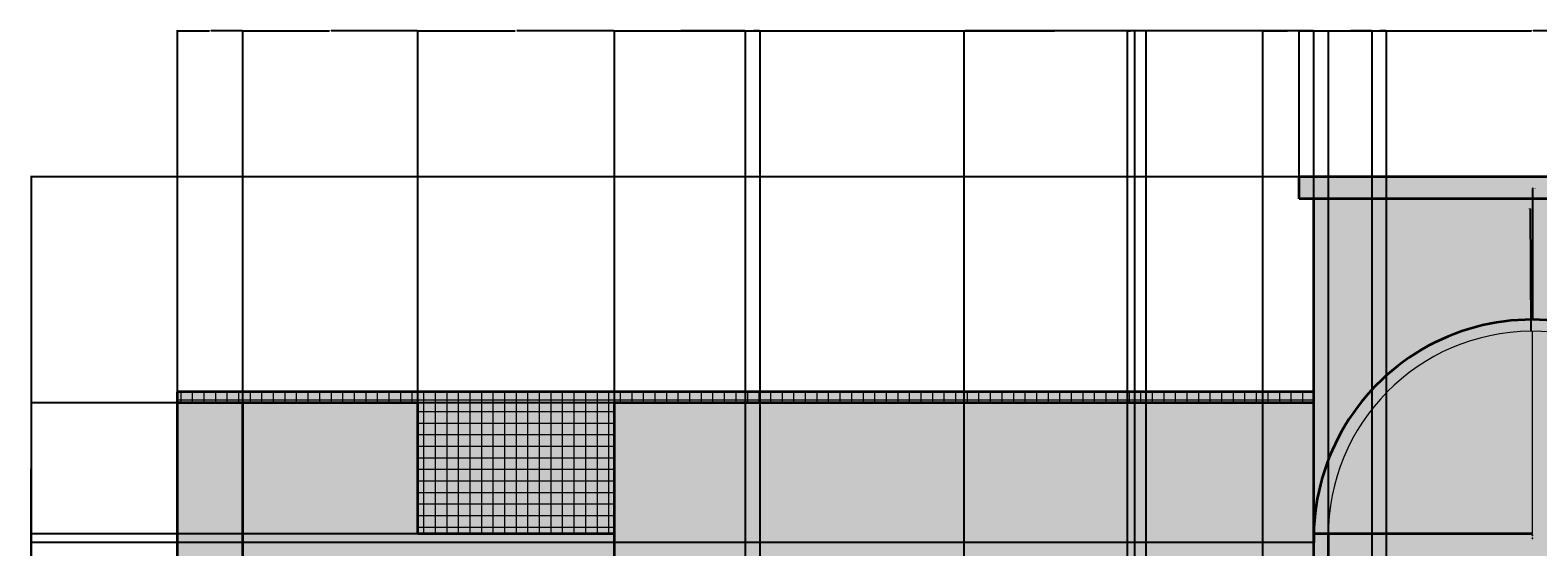
# Model space of a CAD drawing. Units: inches. Extents: x 2794 to 3619, y 522 to 1397.
# Tile 8 of 10: x 2794 to 3208, y 1255 to 1397. Entities that reach past the tile are written whole.
import ezdxf

# ---------------------------------------------------------------- set-up
doc = ezdxf.new("R2010")
doc.units = ezdxf.units.IN
for name, color, linetype, lineweight in [('A-ANNO-DIMS', 2, 'Continuous', 18), ('A-ELEV', 7, 'Continuous', 35), ('A-ELEV-PATT', 8, 'Continuous', 13), ('A-GLAZ', 4, 'Continuous', 18)]:
    doc.layers.add(name, color=color, linetype=linetype, lineweight=lineweight)
doc.styles.get("Standard").update_dxf_attribs({"font": 'arial.ttf'})
doc.dimstyles.get("Standard").update_dxf_attribs({"dimtxt": 0.18, "dimasz": 0.18, "dimexe": 0.18, "dimexo": 0.0625, "dimgap": 0.09, "dimtad": 0, "dimtih": 1, "dimtoh": 1, "dimdec": 4, "dimzin": 0, "dimdsep": 46, "dimtxsty": 'Standard', "dimcen": 0.09, "dimadec": 0, "dimazin": 0, "dimtfac": 1, "dimtdec": 4, "dimtofl": 0, "dimtmove": 0, "dimatfit": 3, "dimfxl": 1, "dimtolj": 1, "dimtzin": 0, "dimarcsym": 0})

# ---------------------------------------------------------------- blocks, each defined once
blk = doc.blocks.new('*D8')
at = {"layer": 'A-ANNO-DIMS', "color": 0, "lineweight": -2, "transparency": 16777216}
for p, q in [((2834.27, 1294.7), (2834.27, 1396.92)), ((2834.45, 1396.74), (2843.06, 1396.74)), ((2852.09, 1396.74), (2843.48, 1396.74)), ((2852.27, 1294.7), (2852.27, 1396.92))]:
    blk.add_line(p, q, dxfattribs=at)
at = {"layer": 'A-ANNO-DIMS', "color": 0, "transparency": 16777216}
for points in [[(2834.45, 1396.77), (2834.45, 1396.71), (2834.27, 1396.74)], [(2852.09, 1396.77), (2852.09, 1396.71), (2852.27, 1396.74)]]:
    blk.add_solid(points, dxfattribs=at)
at = {"layer": 'Defpoints', "color": 0, "transparency": 16777216}
for p in [(2852.27, 1396.74), (2834.27, 1294.64), (2852.27, 1294.64)]:
    blk.add_point(p, dxfattribs=at)
at = {"layer": 'A-ANNO-DIMS', "color": 0, "transparency": 16777216, "insert": (2843.27, 1396.74), "char_height": 0.18, "attachment_point": 5}
blk.add_mtext('\\A1;18', dxfattribs=at)
blk = doc.blocks.new('*D9')
at = {"layer": 'A-ANNO-DIMS', "color": 0, "lineweight": -2, "transparency": 16777216}
for p, q in [((2852.27, 1294.7), (2852.27, 1396.92)), ((2852.45, 1396.74), (2876.04, 1396.74)), ((2900.09, 1396.74), (2876.49, 1396.74)), ((2900.27, 1294.7), (2900.27, 1396.92))]:
    blk.add_line(p, q, dxfattribs=at)
at = {"layer": 'A-ANNO-DIMS', "color": 0, "transparency": 16777216}
for points in [[(2852.45, 1396.77), (2852.45, 1396.71), (2852.27, 1396.74)], [(2900.09, 1396.77), (2900.09, 1396.71), (2900.27, 1396.74)]]:
    blk.add_solid(points, dxfattribs=at)
at = {"layer": 'Defpoints', "color": 0, "transparency": 16777216}
for p in [(2900.27, 1396.74), (2852.27, 1294.64), (2900.27, 1294.64)]:
    blk.add_point(p, dxfattribs=at)
at = {"layer": 'A-ANNO-DIMS', "color": 0, "transparency": 16777216, "insert": (2876.27, 1396.74), "char_height": 0.18, "attachment_point": 5}
blk.add_mtext('\\A1;48', dxfattribs=at)
blk = doc.blocks.new('*D10')
at = {"layer": 'A-ANNO-DIMS', "color": 0, "lineweight": -2, "transparency": 16777216}
for p, q in [((2900.27, 1294.7), (2900.27, 1396.92)), ((2900.45, 1396.74), (2927.05, 1396.74)), ((2954.09, 1396.74), (2927.48, 1396.74)), ((2954.27, 1294.7), (2954.27, 1396.92))]:
    blk.add_line(p, q, dxfattribs=at)
at = {"layer": 'A-ANNO-DIMS', "color": 0, "transparency": 16777216}
for points in [[(2900.45, 1396.77), (2900.45, 1396.71), (2900.27, 1396.74)], [(2954.09, 1396.77), (2954.09, 1396.71), (2954.27, 1396.74)]]:
    blk.add_solid(points, dxfattribs=at)
at = {"layer": 'Defpoints', "color": 0, "transparency": 16777216}
for p in [(2954.27, 1396.74), (2900.27, 1294.64), (2954.27, 1294.64)]:
    blk.add_point(p, dxfattribs=at)
at = {"layer": 'A-ANNO-DIMS', "color": 0, "transparency": 16777216, "insert": (2927.27, 1396.74), "char_height": 0.18, "attachment_point": 5}
blk.add_mtext('\\A1;54', dxfattribs=at)
blk = doc.blocks.new('*D11')
at = {"layer": 'A-ANNO-DIMS', "color": 0, "lineweight": -2, "transparency": 16777216}
for p, q in [((2954.27, 1294.7), (2954.27, 1396.92)), ((2954.45, 1396.74), (3049.99, 1396.74)), ((3146.09, 1396.74), (3050.55, 1396.74)), ((3146.27, 1294.7), (3146.27, 1396.92))]:
    blk.add_line(p, q, dxfattribs=at)
at = {"layer": 'A-ANNO-DIMS', "color": 0, "transparency": 16777216}
for points in [[(2954.45, 1396.77), (2954.45, 1396.71), (2954.27, 1396.74)], [(3146.09, 1396.77), (3146.09, 1396.71), (3146.27, 1396.74)]]:
    blk.add_solid(points, dxfattribs=at)
at = {"layer": 'Defpoints', "color": 0, "transparency": 16777216}
for p in [(3146.27, 1396.74), (2954.27, 1294.64), (3146.27, 1294.64)]:
    blk.add_point(p, dxfattribs=at)
at = {"layer": 'A-ANNO-DIMS', "color": 0, "transparency": 16777216, "insert": (3050.27, 1396.74), "char_height": 0.18, "attachment_point": 5}
blk.add_mtext('\\A1;192', dxfattribs=at)
blk = doc.blocks.new('*D16')
at = {"layer": 'A-ANNO-DIMS', "color": 0, "lineweight": -2, "transparency": 16777216}
for p, q in [((3142.2, 1356.64), (2793.99, 1356.64)), ((2794.17, 1356.46), (2794.17, 959.82)), ((2794.17, 562.82), (2794.17, 959.45)), ((2834.2, 562.64), (2793.99, 562.64))]:
    blk.add_line(p, q, dxfattribs=at)
at = {"layer": 'A-ANNO-DIMS', "color": 0, "transparency": 16777216}
for points in [[(2794.14, 1356.46), (2794.2, 1356.46), (2794.17, 1356.64)], [(2794.14, 562.82), (2794.2, 562.82), (2794.17, 562.64)]]:
    blk.add_solid(points, dxfattribs=at)
at = {"layer": 'Defpoints', "color": 0, "transparency": 16777216}
for p in [(2794.17, 1356.64), (3142.27, 1356.64), (2834.27, 562.64)]:
    blk.add_point(p, dxfattribs=at)
at = {"layer": 'A-ANNO-DIMS', "color": 0, "transparency": 16777216, "insert": (2794.17, 959.64), "char_height": 0.18, "attachment_point": 5}
blk.add_mtext('\\A1;794', dxfattribs=at)
blk = doc.blocks.new('*D26')
at = {"layer": 'A-ANNO-DIMS', "color": 0, "lineweight": -2, "transparency": 16777216}
for p, q in [((2900.2, 1294.64), (2793.99, 1294.64)), ((2794.17, 1294.46), (2794.17, 1276.82)), ((2794.17, 1258.82), (2794.17, 1276.45)), ((2900.2, 1258.64), (2793.99, 1258.64))]:
    blk.add_line(p, q, dxfattribs=at)
at = {"layer": 'A-ANNO-DIMS', "color": 0, "transparency": 16777216}
for points in [[(2794.14, 1294.46), (2794.2, 1294.46), (2794.17, 1294.64)], [(2794.14, 1258.82), (2794.2, 1258.82), (2794.17, 1258.64)]]:
    blk.add_solid(points, dxfattribs=at)
at = {"layer": 'Defpoints', "color": 0, "transparency": 16777216}
for p in [(2794.17, 1294.64), (2900.27, 1294.64), (2900.27, 1258.64)]:
    blk.add_point(p, dxfattribs=at)
at = {"layer": 'A-ANNO-DIMS', "color": 0, "transparency": 16777216, "insert": (2794.17, 1276.64), "char_height": 0.18, "attachment_point": 5}
blk.add_mtext('\\A1;36', dxfattribs=at)
blk = doc.blocks.new('*D27')
at = {"layer": 'A-ANNO-DIMS', "color": 0, "lineweight": -2, "transparency": 16777216}
for p, q in [((2954.2, 1294.64), (2793.99, 1294.64)), ((2794.17, 1294.46), (2794.17, 1261.82)), ((2794.17, 1228.82), (2794.17, 1261.45)), ((2954.2, 1228.64), (2793.99, 1228.64))]:
    blk.add_line(p, q, dxfattribs=at)
at = {"layer": 'A-ANNO-DIMS', "color": 0, "transparency": 16777216}
for points in [[(2794.14, 1294.46), (2794.2, 1294.46), (2794.17, 1294.64)], [(2794.14, 1228.82), (2794.2, 1228.82), (2794.17, 1228.64)]]:
    blk.add_solid(points, dxfattribs=at)
at = {"layer": 'Defpoints', "color": 0, "transparency": 16777216}
for p in [(2794.17, 1294.64), (2954.27, 1294.64), (2954.27, 1228.64)]:
    blk.add_point(p, dxfattribs=at)
at = {"layer": 'A-ANNO-DIMS', "color": 0, "transparency": 16777216, "insert": (2794.17, 1261.64), "char_height": 0.18, "attachment_point": 5}
blk.add_mtext('\\A1;66', dxfattribs=at)
blk = doc.blocks.new('*D28')
at = {"layer": 'A-ANNO-DIMS', "color": 0, "lineweight": -2, "transparency": 16777216}
for p, q in [((2954.27, 832.7), (2954.27, 1396.92)), ((2954.45, 1396.74), (2972.05, 1396.74)), ((2990.09, 1396.74), (2972.48, 1396.74)), ((2990.27, 820.7), (2990.27, 1396.92))]:
    blk.add_line(p, q, dxfattribs=at)
at = {"layer": 'A-ANNO-DIMS', "color": 0, "transparency": 16777216}
for points in [[(2954.45, 1396.77), (2954.45, 1396.71), (2954.27, 1396.74)], [(2990.09, 1396.77), (2990.09, 1396.71), (2990.27, 1396.74)]]:
    blk.add_solid(points, dxfattribs=at)
at = {"layer": 'Defpoints', "color": 0, "transparency": 16777216}
for p in [(2990.27, 1396.74), (2954.27, 832.64), (2990.27, 820.64)]:
    blk.add_point(p, dxfattribs=at)
at = {"layer": 'A-ANNO-DIMS', "color": 0, "transparency": 16777216, "insert": (2972.27, 1396.74), "char_height": 0.18, "attachment_point": 5}
blk.add_mtext('\\A1;36', dxfattribs=at)
blk = doc.blocks.new('*D29')
at = {"layer": 'A-ANNO-DIMS', "color": 0, "lineweight": -2, "transparency": 16777216}
for p, q in [((2990.27, 820.7), (2990.27, 1396.92)), ((2990.45, 1396.74), (2992.11, 1396.74)), ((2994.09, 1396.74), (2992.42, 1396.74)), ((2994.27, 816.7), (2994.27, 1396.92))]:
    blk.add_line(p, q, dxfattribs=at)
at = {"layer": 'A-ANNO-DIMS', "color": 0, "transparency": 16777216}
for points in [[(2990.45, 1396.77), (2990.45, 1396.71), (2990.27, 1396.74)], [(2994.09, 1396.77), (2994.09, 1396.71), (2994.27, 1396.74)]]:
    blk.add_solid(points, dxfattribs=at)
at = {"layer": 'Defpoints', "color": 0, "transparency": 16777216}
for p in [(2994.27, 1396.74), (2990.27, 820.64), (2994.27, 816.64)]:
    blk.add_point(p, dxfattribs=at)
at = {"layer": 'A-ANNO-DIMS', "color": 0, "transparency": 16777216, "insert": (2992.27, 1396.74), "char_height": 0.18, "attachment_point": 5}
blk.add_mtext('\\A1;4', dxfattribs=at)
blk = doc.blocks.new('*D30')
at = {"layer": 'A-ANNO-DIMS', "color": 0, "lineweight": -2, "transparency": 16777216}
for p, q in [((3050.27, 820.7), (3050.27, 1396.92)), ((3050.45, 1396.74), (3075.05, 1396.74)), ((3100.09, 1396.74), (3075.48, 1396.74)), ((3100.27, 820.7), (3100.27, 1396.92))]:
    blk.add_line(p, q, dxfattribs=at)
at = {"layer": 'A-ANNO-DIMS', "color": 0, "transparency": 16777216}
for points in [[(3050.45, 1396.77), (3050.45, 1396.71), (3050.27, 1396.74)], [(3100.09, 1396.77), (3100.09, 1396.71), (3100.27, 1396.74)]]:
    blk.add_solid(points, dxfattribs=at)
at = {"layer": 'Defpoints', "color": 0, "transparency": 16777216}
for p in [(3100.27, 1396.74), (3050.27, 820.64), (3100.27, 820.64)]:
    blk.add_point(p, dxfattribs=at)
at = {"layer": 'A-ANNO-DIMS', "color": 0, "transparency": 16777216, "insert": (3075.27, 1396.74), "char_height": 0.18, "attachment_point": 5}
blk.add_mtext('\\A1;50', dxfattribs=at)
blk = doc.blocks.new('*D31')
at = {"layer": 'A-ANNO-DIMS', "color": 0, "lineweight": -2, "transparency": 16777216}
for p, q in [((3132.27, 820.7), (3132.27, 1396.92)), ((3132.45, 1396.74), (3139.06, 1396.74)), ((3146.09, 1396.74), (3139.48, 1396.74)), ((3146.27, 774.7), (3146.27, 1396.92))]:
    blk.add_line(p, q, dxfattribs=at)
at = {"layer": 'A-ANNO-DIMS', "color": 0, "transparency": 16777216}
for points in [[(3132.45, 1396.77), (3132.45, 1396.71), (3132.27, 1396.74)], [(3146.09, 1396.77), (3146.09, 1396.71), (3146.27, 1396.74)]]:
    blk.add_solid(points, dxfattribs=at)
at = {"layer": 'Defpoints', "color": 0, "transparency": 16777216}
for p in [(3146.27, 1396.74), (3132.27, 820.64), (3146.27, 774.64)]:
    blk.add_point(p, dxfattribs=at)
at = {"layer": 'A-ANNO-DIMS', "color": 0, "transparency": 16777216, "insert": (3139.27, 1396.74), "char_height": 0.18, "attachment_point": 5}
blk.add_mtext('\\A1;14', dxfattribs=at)
blk = doc.blocks.new('*D37')
at = {"layer": 'A-ANNO-DIMS', "color": 0, "lineweight": -2, "transparency": 16777216}
for p, q in [((3095.13, 772.7), (3095.13, 1396.92)), ((3095.31, 1396.74), (3095.98, 1396.74)), ((3096.95, 1396.74), (3096.28, 1396.74)), ((3097.13, 772.7), (3097.13, 1396.92))]:
    blk.add_line(p, q, dxfattribs=at)
at = {"layer": 'A-ANNO-DIMS', "color": 0, "transparency": 16777216}
for points in [[(3095.31, 1396.77), (3095.31, 1396.71), (3095.13, 1396.74)], [(3096.95, 1396.77), (3096.95, 1396.71), (3097.13, 1396.74)]]:
    blk.add_solid(points, dxfattribs=at)
at = {"layer": 'Defpoints', "color": 0, "transparency": 16777216}
for p in [(3097.13, 1396.74), (3095.13, 772.64), (3097.13, 772.64)]:
    blk.add_point(p, dxfattribs=at)
at = {"layer": 'A-ANNO-DIMS', "color": 0, "transparency": 16777216, "insert": (3096.13, 1396.74), "char_height": 0.18, "attachment_point": 5}
blk.add_mtext('\\A1;2', dxfattribs=at)
blk = doc.blocks.new('*D44')
at = {"layer": 'A-ANNO-DIMS', "color": 0, "lineweight": -2, "transparency": 16777216}
for p, q in [((3142.27, 1356.7), (3142.27, 1396.92)), ((3142.45, 1396.74), (3205.99, 1396.74)), ((3270.09, 1396.74), (3206.55, 1396.74)), ((3270.27, 1356.7), (3270.27, 1396.92))]:
    blk.add_line(p, q, dxfattribs=at)
at = {"layer": 'A-ANNO-DIMS', "color": 0, "transparency": 16777216}
for points in [[(3142.45, 1396.77), (3142.45, 1396.71), (3142.27, 1396.74)], [(3270.09, 1396.77), (3270.09, 1396.71), (3270.27, 1396.74)]]:
    blk.add_solid(points, dxfattribs=at)
at = {"layer": 'Defpoints', "color": 0, "transparency": 16777216}
for p in [(3270.27, 1396.74), (3142.27, 1356.64), (3270.27, 1356.64)]:
    blk.add_point(p, dxfattribs=at)
at = {"layer": 'A-ANNO-DIMS', "color": 0, "transparency": 16777216, "insert": (3206.27, 1396.74), "char_height": 0.18, "attachment_point": 5}
blk.add_mtext('\\A1;128', dxfattribs=at)
blk = doc.blocks.new('*D45')
at = {"layer": 'A-ANNO-DIMS', "color": 0, "lineweight": -2, "transparency": 16777216}
for p, q in [((3146.27, 1350.7), (3146.27, 1396.92)), ((3146.45, 1396.74), (3205.99, 1396.74)), ((3266.09, 1396.74), (3206.55, 1396.74)), ((3266.27, 1350.7), (3266.27, 1396.92))]:
    blk.add_line(p, q, dxfattribs=at)
at = {"layer": 'A-ANNO-DIMS', "color": 0, "transparency": 16777216}
for points in [[(3146.45, 1396.77), (3146.45, 1396.71), (3146.27, 1396.74)], [(3266.09, 1396.77), (3266.09, 1396.71), (3266.27, 1396.74)]]:
    blk.add_solid(points, dxfattribs=at)
at = {"layer": 'Defpoints', "color": 0, "transparency": 16777216}
for p in [(3266.27, 1396.74), (3146.27, 1350.64), (3266.27, 1350.64)]:
    blk.add_point(p, dxfattribs=at)
at = {"layer": 'A-ANNO-DIMS', "color": 0, "transparency": 16777216, "insert": (3206.27, 1396.74), "char_height": 0.18, "attachment_point": 5}
blk.add_mtext('\\A1;120', dxfattribs=at)
blk = doc.blocks.new('*D48')
at = {"layer": 'A-ANNO-DIMS', "color": 0, "lineweight": -2, "transparency": 16777216}
for p, q in [((3146.2, 1294.64), (2793.99, 1294.64)), ((2794.17, 1294.46), (2794.17, 1275.62)), ((2794.17, 1256.43), (2794.17, 1275.26)), ((3146.2, 1256.25), (2793.99, 1256.25))]:
    blk.add_line(p, q, dxfattribs=at)
at = {"layer": 'A-ANNO-DIMS', "color": 0, "transparency": 16777216}
for points in [[(2794.14, 1294.46), (2794.2, 1294.46), (2794.17, 1294.64)], [(2794.14, 1256.43), (2794.2, 1256.43), (2794.17, 1256.25)]]:
    blk.add_solid(points, dxfattribs=at)
at = {"layer": 'Defpoints', "color": 0, "transparency": 16777216}
for p in [(2794.17, 1294.64), (3146.27, 1294.64), (3146.27, 1256.25)]:
    blk.add_point(p, dxfattribs=at)
at = {"layer": 'A-ANNO-DIMS', "color": 0, "transparency": 16777216, "insert": (2794.17, 1275.44), "char_height": 0.18, "attachment_point": 5}
blk.add_mtext('\\A1;38.39', dxfattribs=at)
blk = doc.blocks.new('*D49')
at = {"layer": 'A-ANNO-DIMS', "color": 0, "lineweight": -2, "transparency": 16777216}
for p, q in [((3146.27, 1256.19), (3146.27, 522.36)), ((3150.27, 1254.57), (3150.27, 522.36)), ((3146.45, 522.54), (3148.11, 522.54)), ((3150.09, 522.54), (3148.42, 522.54))]:
    blk.add_line(p, q, dxfattribs=at)
at = {"layer": 'A-ANNO-DIMS', "color": 0, "transparency": 16777216}
for points in [[(3146.45, 522.57), (3146.45, 522.51), (3146.27, 522.54)], [(3150.09, 522.57), (3150.09, 522.51), (3150.27, 522.54)]]:
    blk.add_solid(points, dxfattribs=at)
at = {"layer": 'Defpoints', "color": 0, "transparency": 16777216}
for p in [(3146.27, 1256.25), (3150.27, 1254.64), (3150.27, 522.54)]:
    blk.add_point(p, dxfattribs=at)
at = {"layer": 'A-ANNO-DIMS', "color": 0, "transparency": 16777216, "insert": (3148.27, 522.54), "char_height": 0.18, "attachment_point": 5}
blk.add_mtext('\\A1;4', dxfattribs=at)
blk = doc.blocks.new('*D56')
at = {"layer": 'A-ANNO-DIMS', "color": 0, "lineweight": -2, "transparency": 16777216}
for p, q in [((3162.27, 664.7), (3162.27, 1396.92)), ((3162.45, 1396.74), (3206.05, 1396.74)), ((3250.09, 1396.74), (3206.49, 1396.74)), ((3250.27, 664.7), (3250.27, 1396.92))]:
    blk.add_line(p, q, dxfattribs=at)
at = {"layer": 'A-ANNO-DIMS', "color": 0, "transparency": 16777216}
for points in [[(3162.45, 1396.77), (3162.45, 1396.71), (3162.27, 1396.74)], [(3250.09, 1396.77), (3250.09, 1396.71), (3250.27, 1396.74)]]:
    blk.add_solid(points, dxfattribs=at)
at = {"layer": 'Defpoints', "color": 0, "transparency": 16777216}
for p in [(3250.27, 1396.74), (3162.27, 664.64), (3250.27, 664.64)]:
    blk.add_point(p, dxfattribs=at)
at = {"layer": 'A-ANNO-DIMS', "color": 0, "transparency": 16777216, "insert": (3206.27, 1396.74), "char_height": 0.18, "attachment_point": 5}
blk.add_mtext('\\A1;88', dxfattribs=at)
blk = doc.blocks.new('*D57')
at = {"layer": 'A-ANNO-DIMS', "color": 0, "lineweight": -2, "transparency": 16777216}
for p, q in [((3162.27, 664.7), (3162.27, 1396.92)), ((3162.45, 1396.74), (3164.11, 1396.74)), ((3166.09, 1396.74), (3164.42, 1396.74)), ((3166.27, 660.7), (3166.27, 1396.92))]:
    blk.add_line(p, q, dxfattribs=at)
at = {"layer": 'A-ANNO-DIMS', "color": 0, "transparency": 16777216}
for points in [[(3162.45, 1396.77), (3162.45, 1396.71), (3162.27, 1396.74)], [(3166.09, 1396.77), (3166.09, 1396.71), (3166.27, 1396.74)]]:
    blk.add_solid(points, dxfattribs=at)
at = {"layer": 'Defpoints', "color": 0, "transparency": 16777216}
for p in [(3166.27, 1396.74), (3162.27, 664.64), (3166.27, 660.64)]:
    blk.add_point(p, dxfattribs=at)
at = {"layer": 'A-ANNO-DIMS', "color": 0, "transparency": 16777216, "insert": (3164.27, 1396.74), "char_height": 0.18, "attachment_point": 5}
blk.add_mtext('\\A1;4', dxfattribs=at)
blk = doc.blocks.new('*D58')
at = {"layer": 'A-ANNO-DIMS', "color": 0, "lineweight": -2, "transparency": 16777216}
for p, q in [((3150.27, 580.7), (3150.27, 1396.92)), ((3150.45, 1396.74), (3156.06, 1396.74)), ((3162.09, 1396.74), (3156.48, 1396.74)), ((3162.27, 664.7), (3162.27, 1396.92))]:
    blk.add_line(p, q, dxfattribs=at)
at = {"layer": 'A-ANNO-DIMS', "color": 0, "transparency": 16777216}
for points in [[(3150.45, 1396.77), (3150.45, 1396.71), (3150.27, 1396.74)], [(3162.09, 1396.77), (3162.09, 1396.71), (3162.27, 1396.74)]]:
    blk.add_solid(points, dxfattribs=at)
at = {"layer": 'Defpoints', "color": 0, "transparency": 16777216}
for p in [(3162.27, 1396.74), (3162.27, 664.64), (3150.27, 580.64)]:
    blk.add_point(p, dxfattribs=at)
at = {"layer": 'A-ANNO-DIMS', "color": 0, "transparency": 16777216, "insert": (3156.27, 1396.74), "char_height": 0.18, "attachment_point": 5}
blk.add_mtext('\\A1;12', dxfattribs=at)
blk = doc.blocks.new('*D64')
at = {"layer": 'A-ANNO-DIMS', "color": 0, "lineweight": -2, "transparency": 16777216}
for p, q in [((3206.45, 1353.46), (3206.27, 1353.46)), ((3206.27, 1353.46), (3206.27, 1317.63)), ((3206.18, 1257.44), (3206.36, 1257.44)), ((3206.27, 1257.35), (3206.27, 1257.53))]:
    blk.add_line(p, q, dxfattribs=at)
at = {"layer": 'A-ANNO-DIMS', "color": 0, "transparency": 16777216}
blk.add_solid([(3206.24, 1317.63), (3206.3, 1317.63), (3206.27, 1317.45)], dxfattribs=at)
at = {"layer": 'Defpoints', "color": 0, "transparency": 16777216}
for p in [(3206.27, 1317.45), (3206.27, 1257.44)]:
    blk.add_point(p, dxfattribs=at)
at = {"layer": 'A-ANNO-DIMS', "color": 0, "transparency": 16777216, "insert": (3206.91, 1353.46), "char_height": 0.18, "attachment_point": 5}
blk.add_mtext('\\A1;R60.01', dxfattribs=at)
blk = doc.blocks.new('*D65')
at = {"layer": 'A-ANNO-DIMS', "color": 0, "lineweight": -2, "transparency": 16777216}
for p, q in [((3205.48, 1347.85), (3205.66, 1347.85)), ((3205.66, 1347.85), (3205.88, 1314.43)), ((3206.27, 1258.16), (3206.27, 1258.34)), ((3206.18, 1258.25), (3206.36, 1258.25))]:
    blk.add_line(p, q, dxfattribs=at)
at = {"layer": 'A-ANNO-DIMS', "color": 0, "transparency": 16777216}
blk.add_solid([(3205.91, 1314.43), (3205.85, 1314.43), (3205.89, 1314.25)], dxfattribs=at)
at = {"layer": 'Defpoints', "color": 0, "transparency": 16777216}
for p in [(3205.89, 1314.25), (3206.27, 1258.25)]:
    blk.add_point(p, dxfattribs=at)
at = {"layer": 'A-ANNO-DIMS', "color": 0, "transparency": 16777216, "insert": (3205.17, 1347.85), "char_height": 0.18, "attachment_point": 5}
blk.add_mtext('\\A1;R56', dxfattribs=at)

msp = doc.modelspace()

# ---------------------------------------------------------------- hatches: boundary and pattern name
at = {"layer": 'A-ELEV-PATT', "transparency": 33554687}
h = msp.add_hatch(color=256, dxfattribs=at)
h.dxf.hatch_style = 1
h.paths.add_polyline_path([(3270.2659, 1356.6351), (3142.2659, 1356.6351), (3142.2659, 1350.6351), (3266.2659, 1350.6351), (3270.2659, 1350.6351)])
h.paths.add_polyline_path([(3266.2659, 1350.6351), (3262.2659, 1350.6351), (3262.2659, 1279.0155, -0.0871789), (3266.2659, 1258.6351)])
h.paths.add_polyline_path([(3150.2659, 1350.6351), (3146.2659, 1350.6351), (3146.2659, 1258.6351, -0.0871789), (3150.2659, 1279.0155)])
h = msp.add_hatch(color=256, dxfattribs=at)
h.dxf.hatch_style = 1
h.paths.add_polyline_path([(3262.2659, 1350.6351), (3150.2659, 1350.6351), (3150.2659, 1279.0155, -0.68639605), (3262.2659, 1279.0155)])
h.paths.add_polyline_path([(3210.2659, 1314.1121), (3210.2659, 1258.6351), (3262.2659, 1258.6351, 0.39146256)])
h.paths.add_polyline_path([(3206.2659, 1314.2551, 0.41222069), (3150.2659, 1258.6351), (3206.2659, 1258.6351)])
h.paths.add_polyline_path([(3262.2659, 1254.6351), (3210.2659, 1254.6351), (3210.2659, 1216.6351), (3262.2659, 1216.6351)])
h.paths.add_polyline_path([(3206.2659, 1254.6351), (3150.2659, 1254.6351), (3150.2659, 1216.6351), (3206.2659, 1216.6351)])
h.paths.add_polyline_path([(3262.2659, 1212.6351), (3210.2659, 1212.6351), (3210.2659, 1186.6351), (3262.2659, 1186.6351)])
h.paths.add_polyline_path([(3206.2659, 1212.6351), (3150.2659, 1212.6351), (3150.2659, 1186.6351), (3206.2659, 1186.6351)])
h.paths.add_polyline_path([(3206.2659, 1182.6351), (3150.2659, 1182.6351), (3150.2659, 1156.6351), (3206.2659, 1156.6351)])
h.paths.add_polyline_path([(3262.2659, 1182.6351), (3210.2659, 1182.6351), (3210.2659, 1156.6351), (3262.2659, 1156.6351)])
h.paths.add_polyline_path([(3262.2659, 1152.6351), (3210.2659, 1152.6351), (3210.2659, 1126.6351), (3262.2659, 1126.6351)])
h.paths.add_polyline_path([(3206.2659, 1152.6351), (3150.2659, 1152.6351), (3150.2659, 1126.6351), (3206.2659, 1126.6351)])
h.paths.add_polyline_path([(3262.2659, 1122.6351), (3210.2659, 1122.6351), (3210.2659, 1096.6351), (3262.2659, 1096.6351)])
h.paths.add_polyline_path([(3206.2659, 1122.6351), (3150.2659, 1122.6351), (3150.2659, 1096.6351), (3206.2659, 1096.6351)])
h.paths.add_polyline_path([(3206.2659, 1092.6351), (3150.2659, 1092.6351), (3150.2659, 1066.6351), (3206.2659, 1066.6351)])
h.paths.add_polyline_path([(3262.2659, 1092.6351), (3210.2659, 1092.6351), (3210.2659, 1066.6351), (3262.2659, 1066.6351)])
h.paths.add_polyline_path([(3262.2659, 1062.6351), (3210.2659, 1062.6351), (3210.2659, 1036.6351), (3262.2659, 1036.6351)])
h.paths.add_polyline_path([(3206.2659, 1062.6351), (3150.2659, 1062.6351), (3150.2659, 1036.6351), (3206.2659, 1036.6351)])
h.paths.add_polyline_path([(3206.2659, 1032.6351), (3150.2659, 1032.6351), (3150.2659, 1006.6351), (3206.2659, 1006.6351)])
h.paths.add_polyline_path([(3262.2659, 1032.6351), (3210.2659, 1032.6351), (3210.2659, 1006.6351), (3262.2659, 1006.6351)])
h.paths.add_polyline_path([(3262.2659, 1002.6351), (3210.2659, 1002.6351), (3210.2659, 976.6351), (3262.2659, 976.6351)])
h.paths.add_polyline_path([(3206.2659, 1002.6351), (3150.2659, 1002.6351), (3150.2659, 976.6351), (3206.2659, 976.6351)])
h.paths.add_polyline_path([(3206.2659, 972.6351), (3150.2659, 972.6351), (3150.2659, 946.6351), (3206.2659, 946.6351)])
h.paths.add_polyline_path([(3206.2659, 942.6351), (3150.2659, 942.6351), (3150.2659, 916.6351), (3206.2659, 916.6351)])
h.paths.add_polyline_path([(3262.2659, 942.6351), (3210.2659, 942.6351), (3210.2659, 916.6351), (3262.2659, 916.6351)])
h.paths.add_polyline_path([(3262.2659, 972.6351), (3210.2659, 972.6351), (3210.2659, 946.6351), (3262.2659, 946.6351)])
h.paths.add_polyline_path([(3262.2659, 912.6351), (3210.2659, 912.6351), (3210.2659, 886.6351), (3262.2659, 886.6351)])
h.paths.add_polyline_path([(3206.2659, 912.6351), (3150.2659, 912.6351), (3150.2659, 886.6351), (3206.2659, 886.6351)])
h.paths.add_polyline_path([(3206.2659, 882.6351), (3150.2659, 882.6351), (3150.2659, 856.6351), (3206.2659, 856.6351)])
h.paths.add_polyline_path([(3262.2659, 882.6351), (3210.2659, 882.6351), (3210.2659, 856.6351), (3262.2659, 856.6351)])
h.paths.add_polyline_path([(3262.2659, 852.6351), (3210.2659, 852.6351), (3210.2659, 826.6351), (3262.2659, 826.6351)])
h.paths.add_polyline_path([(3206.2659, 852.6351), (3150.2659, 852.6351), (3150.2659, 826.6351), (3206.2659, 826.6351)])
h.paths.add_polyline_path([(3206.2659, 822.6351), (3150.2659, 822.6351), (3150.2659, 796.6351), (3206.2659, 796.6351)])
h.paths.add_polyline_path([(3262.2659, 822.6351), (3210.2659, 822.6351), (3210.2659, 796.6351), (3262.2659, 796.6351)])
h.paths.add_polyline_path([(3262.2659, 792.6351), (3210.2659, 792.6351), (3210.2659, 766.6351), (3262.2659, 766.6351)])
h.paths.add_polyline_path([(3206.2659, 792.6351), (3150.2659, 792.6351), (3150.2659, 766.6351), (3206.2659, 766.6351)])
h.paths.add_polyline_path([(3206.2659, 762.6351), (3150.2659, 762.6351), (3150.2659, 736.6351), (3206.2659, 736.6351)])
h.paths.add_polyline_path([(3206.2659, 732.6351), (3150.2659, 732.6351), (3150.2659, 706.6351), (3206.2659, 706.6351)])
h.paths.add_polyline_path([(3262.2659, 732.6351), (3210.2659, 732.6351), (3210.2659, 706.6351), (3262.2659, 706.6351)])
h.paths.add_polyline_path([(3262.2659, 762.6351), (3210.2659, 762.6351), (3210.2659, 736.6351), (3262.2659, 736.6351)])
h = msp.add_hatch(color=256, dxfattribs=at)
h.dxf.hatch_style = 1
h.paths.add_polyline_path([(3146.2659, 1258.6351), (3150.2659, 1258.6351, -0.9932142), (3262.2659, 1258.6351), (3262.2659, 1279.0155, 0.82281137)])
h = msp.add_hatch(color=256, dxfattribs=at)
h.dxf.hatch_style = 1
h.paths.add_polyline_path([(3266.2659, 1258.6351, 0.98030963), (3146.2659, 1258.6351), (3150.2659, 1258.6351, -0.9932142), (3262.2659, 1258.6351), (3262.2659, 1228.6351), (3266.2659, 1228.6351)])
h = msp.add_hatch(color=256, dxfattribs=at)
h.dxf.hatch_style = 1
h.paths.add_polyline_path([(3150.2659, 1257.8725, -0.00340445), (3150.2659, 1258.6351), (3146.2659, 1258.6351), (3146.2659, 1228.6351), (3150.2659, 1228.6351)])
h.paths.add_polyline_path([(3262.2659, 1258.6351), (3210.2659, 1258.6351), (3210.2659, 1314.1121, 0.01787385), (3206.2659, 1314.2551), (3206.2659, 1258.6351), (3150.2659, 1258.6351), (3150.2659, 1254.6351), (3206.2659, 1254.6351), (3206.2659, 1216.6351), (3150.2659, 1216.6351), (3150.2659, 1212.6351), (3206.2659, 1212.6351), (3206.2659, 1186.6351), (3150.2659, 1186.6351), (3150.2659, 1182.6351), (3206.2659, 1182.6351), (3206.2659, 1156.6351), (3150.2659, 1156.6351), (3150.2659, 1152.6351), (3206.2659, 1152.6351), (3206.2659, 1126.6351), (3150.2659, 1126.6351), (3150.2659, 1122.6351), (3206.2659, 1122.6351), (3206.2659, 1096.6351), (3150.2659, 1096.6351), (3150.2659, 1092.6351), (3206.2659, 1092.6351), (3206.2659, 1066.6351), (3150.2659, 1066.6351), (3150.2659, 1062.6351), (3206.2659, 1062.6351), (3206.2659, 1036.6351), (3150.2659, 1036.6351), (3150.2659, 1032.6351), (3206.2659, 1032.6351), (3206.2659, 1006.6351), (3150.2659, 1006.6351), (3150.2659, 1002.6351), (3206.2659, 1002.6351), (3206.2659, 976.6351), (3150.2659, 976.6351), (3150.2659, 972.6351), (3206.2659, 972.6351), (3206.2659, 946.6351), (3150.2659, 946.6351), (3150.2659, 942.6351), (3206.2659, 942.6351), (3206.2659, 916.6351), (3150.2659, 916.6351), (3150.2659, 912.6351), (3206.2659, 912.6351), (3206.2659, 886.6351), (3150.2659, 886.6351), (3150.2659, 882.6351), (3206.2659, 882.6351), (3206.2659, 856.6351), (3150.2659, 856.6351), (3150.2659, 852.6351), (3206.2659, 852.6351), (3206.2659, 826.6351), (3150.2659, 826.6351), (3150.2659, 822.6351), (3206.2659, 822.6351), (3206.2659, 796.6351), (3150.2659, 796.6351), (3150.2659, 792.6351), (3206.2659, 792.6351), (3206.2659, 766.6351), (3150.2659, 766.6351), (3150.2659, 762.6351), (3206.2659, 762.6351), (3206.2659, 736.6351), (3150.2659, 736.6351), (3150.2659, 732.6351), (3206.2659, 732.6351), (3206.2659, 706.6351), (3150.2659, 706.6351), (3150.2659, 702.6351), (3262.2659, 702.6351), (3262.2659, 706.6351), (3210.2659, 706.6351), (3210.2659, 732.6351), (3262.2659, 732.6351), (3262.2659, 736.6351), (3210.2659, 736.6351), (3210.2659, 762.6351), (3262.2659, 762.6351), (3262.2659, 766.6351), (3210.2659, 766.6351), (3210.2659, 792.6351), (3262.2659, 792.6351), (3262.2659, 796.6351), (3210.2659, 796.6351), (3210.2659, 822.6351), (3262.2659, 822.6351), (3262.2659, 826.6351), (3210.2659, 826.6351), (3210.2659, 852.6351), (3262.2659, 852.6351), (3262.2659, 856.6351), (3210.2659, 856.6351), (3210.2659, 882.6351), (3262.2659, 882.6351), (3262.2659, 886.6351), (3210.2659, 886.6351), (3210.2659, 912.6351), (3262.2659, 912.6351), (3262.2659, 916.6351), (3210.2659, 916.6351), (3210.2659, 942.6351), (3262.2659, 942.6351), (3262.2659, 946.6351), (3210.2659, 946.6351), (3210.2659, 972.6351), (3262.2659, 972.6351), (3262.2659, 976.6351), (3210.2659, 976.6351), (3210.2659, 1002.6351), (3262.2659, 1002.6351), (3262.2659, 1006.6351), (3210.2659, 1006.6351), (3210.2659, 1032.6351), (3262.2659, 1032.6351), (3262.2659, 1036.6351), (3210.2659, 1036.6351), (3210.2659, 1062.6351), (3262.2659, 1062.6351), (3262.2659, 1066.6351), (3210.2659, 1066.6351), (3210.2659, 1092.6351), (3262.2659, 1092.6351), (3262.2659, 1096.6351), (3210.2659, 1096.6351), (3210.2659, 1122.6351), (3262.2659, 1122.6351), (3262.2659, 1126.6351), (3210.2659, 1126.6351), (3210.2659, 1152.6351), (3262.2659, 1152.6351), (3262.2659, 1156.6351), (3210.2659, 1156.6351), (3210.2659, 1182.6351), (3262.2659, 1182.6351), (3262.2659, 1186.6351), (3210.2659, 1186.6351), (3210.2659, 1212.6351), (3262.2659, 1212.6351), (3262.2659, 1216.6351), (3210.2659, 1216.6351), (3210.2659, 1254.6351), (3262.2659, 1254.6351)])
at = {"layer": 'A-ELEV-PATT'}
h = msp.add_hatch(dxfattribs=at)
h.set_pattern_fill('NET', color=256)
h.paths.add_polyline_path([(2834.2659, 1297.6351), (2834.2659, 1294.6351), (2900.2659, 1294.6351), (2900.2659, 1258.6351), (2954.2659, 1258.6351), (2954.2659, 1294.6351), (3146.2659, 1294.6351), (3146.2659, 1297.6351)])
h.paths.add_polyline_path([(3512.2659, 1258.6351), (3512.2659, 1294.6351), (3578.2659, 1294.6351), (3578.2659, 1297.6351), (3266.2659, 1297.6351), (3266.2659, 1294.6351), (3458.2659, 1294.6351), (3458.2659, 1258.6351)])
at = {"layer": 'A-ELEV-PATT', "transparency": 33554687}
h = msp.add_hatch(color=256, dxfattribs=at)
h.dxf.hatch_style = 1
h.paths.add_polyline_path([(2834.2659, 1297.6351), (2834.2659, 1294.6351), (2900.2659, 1294.6351), (2900.2659, 1258.6351), (2954.2659, 1258.6351), (2954.2659, 1294.6351), (3146.2659, 1294.6351), (3146.2659, 1297.6351)])
h = msp.add_hatch(color=256, dxfattribs=at)
h.dxf.hatch_style = 1
h.paths.add_polyline_path([(3578.2659, 1294.6351), (3560.2659, 1294.6351), (3560.2659, 642.6351), (3578.2659, 642.6351)])
h.paths.add_polyline_path([(2852.2659, 1294.6351), (2834.2659, 1294.6351), (2834.2659, 642.6351), (2852.2659, 642.6351)])
h = msp.add_hatch(color=256, dxfattribs=at)
h.dxf.hatch_style = 1
h.paths.add_polyline_path([(2852.2659, 1294.6351), (2834.2659, 1294.6351), (2834.2659, 562.6351), (2852.2659, 562.6351)])
h.paths.add_polyline_path([(3578.2659, 1294.6351), (3560.2659, 1294.6351), (3560.2659, 562.6351), (3578.2659, 562.6351)])
h = msp.add_hatch(color=256, dxfattribs=at)
h.dxf.hatch_style = 1
h.paths.add_polyline_path([(2852.2659, 1246.6351), (2954.2659, 1246.6351), (2954.2659, 1258.6351), (2900.2659, 1258.6351), (2900.2659, 1294.6351), (2852.2659, 1294.6351)])
h.paths.add_polyline_path([(3512.2659, 1294.6351), (3512.2659, 1258.6351), (3458.2659, 1258.6351), (3458.2659, 1246.6351), (3560.2659, 1246.6351), (3560.2659, 1294.6351)])
h.paths.add_polyline_path([(2954.2659, 1114.6351), (2954.2659, 1126.6351), (2852.2659, 1126.6351), (2852.2659, 1114.6351)])
h.paths.add_polyline_path([(3560.2659, 1114.6351), (3560.2659, 1126.6351), (3458.2659, 1126.6351), (3458.2659, 1114.6351)])
h.paths.add_polyline_path([(3560.2659, 982.6351), (3560.2659, 994.6351), (3458.2659, 994.6351), (3458.2659, 982.6351)])
h.paths.add_polyline_path([(2954.2659, 982.6351), (2954.2659, 994.6351), (2852.2659, 994.6351), (2852.2659, 982.6351)])
h.paths.add_polyline_path([(2852.2659, 862.6351), (2852.2659, 850.6351), (2954.2659, 850.6351), (2954.2659, 862.6351)])
h.paths.add_polyline_path([(2852.2659, 730.6351), (2852.2659, 718.6351), (2954.2659, 718.6351), (2954.2659, 730.6351)])
h.paths.add_polyline_path([(3560.2659, 718.6351), (3560.2659, 730.6351), (3458.2659, 730.6351), (3458.2659, 718.6351)])
h.paths.add_polyline_path([(3560.2659, 850.6351), (3560.2659, 862.6351), (3458.2659, 862.6351), (3458.2659, 850.6351)])
h = msp.add_hatch(color=256, dxfattribs=at)
h.dxf.hatch_style = 1
h.paths.add_polyline_path([(3146.2659, 1096.6351), (3146.2659, 1126.6351), (2954.2659, 1126.6351), (2954.2659, 1096.6351)])
h.paths.add_polyline_path([(3458.2659, 1096.6351), (3458.2659, 1126.6351), (3266.2659, 1126.6351), (3266.2659, 1096.6351)])
h.paths.add_polyline_path([(3458.2659, 964.6351), (3458.2659, 994.6351), (3266.2659, 994.6351), (3266.2659, 964.6351)])
h.paths.add_polyline_path([(3146.2659, 964.6351), (3146.2659, 994.6351), (2954.2659, 994.6351), (2954.2659, 964.6351)])
h.paths.add_polyline_path([(3458.2659, 832.6351), (3458.2659, 862.6351), (3266.2659, 862.6351), (3266.2659, 832.6351)])
h.paths.add_polyline_path([(3146.2659, 832.6351), (3146.2659, 862.6351), (2954.2659, 862.6351), (2954.2659, 832.6351)])
h.paths.add_polyline_path([(3458.2659, 700.6351), (3458.2659, 730.6351), (3266.2659, 730.6351), (3266.2659, 700.6351)])
h.paths.add_polyline_path([(3146.2659, 700.6351), (3146.2659, 730.6351), (2954.2659, 730.6351), (2954.2659, 700.6351)])
h.paths.add_polyline_path([(3266.2659, 1294.6351), (3266.2659, 1258.6351), (3266.2659, 1228.6351), (3458.2659, 1228.6351), (3458.2659, 1294.6351)])
h.paths.add_polyline_path([(3146.2659, 1228.6351), (3146.2659, 1256.2485, -0.00994307), (3146.2659, 1258.6351), (3146.2659, 1294.6351), (2954.2659, 1294.6351), (2954.2659, 1228.6351)])

# ---------------------------------------------------------------- linework, layer by layer
at = {"layer": 'A-ELEV'}
for p, q in [((3142.2659, 1350.6351), (3142.2659, 1356.6351)), ((3270.2659, 1356.6351), (3142.2659, 1356.6351)), ((3266.2659, 1350.6351), (3142.2659, 1350.6351)), ((3146.2659, 1258.6351), (3146.2659, 1350.6351)), ((3163.6918, 1350.6351), (3146.2659, 1350.6351)), ((2834.2659, 562.6351), (2834.2659, 1297.6351)), ((3146.2659, 1297.6351), (2834.2659, 1297.6351)), ((2900.2659, 1294.6351), (2834.2659, 1294.6351)), ((2852.2659, 562.6351), (2852.2659, 1294.6351)), ((2900.2659, 1258.6351), (2900.2659, 1294.6351)), ((2954.2659, 598.6351), (2954.2659, 1294.6351)), ((3146.2659, 1294.6351), (2954.2659, 1294.6351)), ((2954.2659, 1258.6351), (2900.2659, 1258.6351)), ((3146.2659, 598.6351), (3146.2659, 1258.6351)), ((3206.2659, 1258.6351), (3146.2659, 1258.6351)), ((3150.2659, 598.6351), (3150.2659, 1258.6351))]:
    msp.add_line(p, q, dxfattribs=at)
msp.add_arc((3206.2659, 1257.4418), 60.0119, 358.860645, 181.139355, dxfattribs=at)
at = {"layer": 'A-GLAZ'}
for p, q in [((3150.2659, 1279.0155), (3150.2659, 1350.6351)), ((3206.2659, 1314.2194), (3206.2659, 1258.6351))]:
    msp.add_line(p, q, dxfattribs=at)
msp.add_arc((3206.2659, 1258.2538), 56.0013, 0.39012, 180.39012, dxfattribs=at)

# ---------------------------------------------------------------- dimensions: what is measured, and where the dimension line sits
at = {"layer": 'A-ANNO-DIMS'}
for base, p1, p2, picture, middle in [((2852.2659, 1396.7351), (2834.2659, 1294.6351), (2852.2659, 1294.6351), '*D8', (2843.2659, 1396.7351)), ((2900.2659, 1396.7351), (2852.2659, 1294.6351), (2900.2659, 1294.6351), '*D9', (2876.2659, 1396.7351)), ((2954.2659, 1396.7351), (2900.2659, 1294.6351), (2954.2659, 1294.6351), '*D10', (2927.2659, 1396.7351)), ((3146.2659, 1396.7351), (2954.2659, 1294.6351), (3146.2659, 1294.6351), '*D11', (3050.2659, 1396.7351)), ((2990.2659, 1396.7351), (2954.2659, 832.6351), (2990.2659, 820.6351), '*D28', (2972.2659, 1396.7351)), ((2994.2659, 1396.7351), (2990.2659, 820.6351), (2994.2659, 816.6351), '*D29', (2992.2659, 1396.7351)), ((3100.2659, 1396.7351), (3050.2659, 820.6351), (3100.2659, 820.6351), '*D30', (3075.2659, 1396.7351)), ((3097.1329, 1396.7351), (3095.1329, 772.6351), (3097.1329, 772.6351), '*D37', (3096.1329, 1396.7351)), ((3146.2659, 1396.7351), (3132.2659, 820.6351), (3146.2659, 774.6351), '*D31', (3139.2659, 1396.7351)), ((3270.2659, 1396.7351), (3142.2659, 1356.6351), (3270.2659, 1356.6351), '*D44', (3206.2659, 1396.7351)), ((3266.2659, 1396.7351), (3146.2659, 1350.6351), (3266.2659, 1350.6351), '*D45', (3206.2659, 1396.7351)), ((3162.2659, 1396.7351), (3150.2659, 580.6351), (3162.2659, 664.6351), '*D58', (3156.2659, 1396.7351)), ((3250.2659, 1396.7351), (3162.2659, 664.6351), (3250.2659, 664.6351), '*D56', (3206.2659, 1396.7351)), ((3166.2659, 1396.7351), (3162.2659, 664.6351), (3166.2659, 660.6351), '*D57', (3164.2659, 1396.7351)), ((3150.2659, 522.5351), (3146.2659, 1256.2485), (3150.2659, 1254.6351), '*D49', (3148.2659, 522.5351))]:
    dim = msp.add_linear_dim(base=base, p1=p1, p2=p2, dimstyle='Standard', override={"dimdec": 0, "dimlfac": 1, "dimrnd": 0, "dimzin": 0, "dimdsep": 46, "dimlunit": 2}, dxfattribs=at)
    dim.commit()
    dim.dimension.update_dxf_attribs({"geometry": picture, "text_midpoint": middle})
for base, p1, p2, override, picture, middle in [((2794.1659, 1356.6351), (2834.2659, 562.6351), (3142.2659, 1356.6351), {"dimdec": 0, "dimlfac": 1, "dimrnd": 0, "dimzin": 0, "dimdsep": 46, "dimlunit": 2}, '*D16', (2794.1659, 959.6351)), ((2794.1659, 1294.6351), (3146.2659, 1256.2485), (3146.2659, 1294.6351), {"dimdec": 2, "dimlfac": 1, "dimrnd": 0, "dimzin": 0, "dimdsep": 46, "dimlunit": 2}, '*D48', (2794.1659, 1275.4418)), ((2794.1659, 1294.6351), (2900.2659, 1258.6351), (2900.2659, 1294.6351), {"dimdec": 0, "dimlfac": 1, "dimrnd": 0, "dimzin": 0, "dimdsep": 46, "dimlunit": 2}, '*D26', (2794.1659, 1276.6351)), ((2794.1659, 1294.6351), (2954.2659, 1228.6351), (2954.2659, 1294.6351), {"dimdec": 0, "dimlfac": 1, "dimrnd": 0, "dimzin": 0, "dimdsep": 46, "dimlunit": 2}, '*D27', (2794.1659, 1261.6351))]:
    dim = msp.add_linear_dim(base=base, p1=p1, p2=p2, angle=90, dimstyle='Standard', override=override, dxfattribs=at)
    dim.commit()
    dim.dimension.update_dxf_attribs({"geometry": picture, "text_midpoint": middle})
for center, mpoint, override, picture, middle in [((3206.2659, 1257.4418), (3206.266, 1317.4537), {"dimdec": 2, "dimlfac": 1, "dimrnd": 0, "dimzin": 0, "dimdsep": 46, "dimlunit": 2}, '*D64', (3206.9086, 1353.4608)), ((3206.2659, 1258.2538), (3205.885, 1314.2538), {"dimdec": 0, "dimlfac": 1, "dimrnd": 0, "dimzin": 0, "dimdsep": 46, "dimlunit": 2}, '*D65', (3205.1715, 1347.8538))]:
    dim = msp.add_radius_dim(center=center, mpoint=mpoint, dimstyle='Standard', override=override, dxfattribs=at)
    dim.commit()
    dim.dimension.update_dxf_attribs({"geometry": picture, "text_midpoint": middle, "dimtype": 164})

doc.saveas('drawing.dxf')
